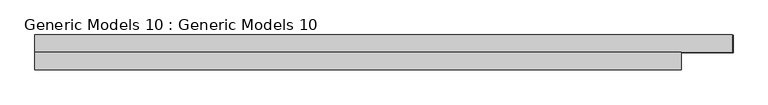
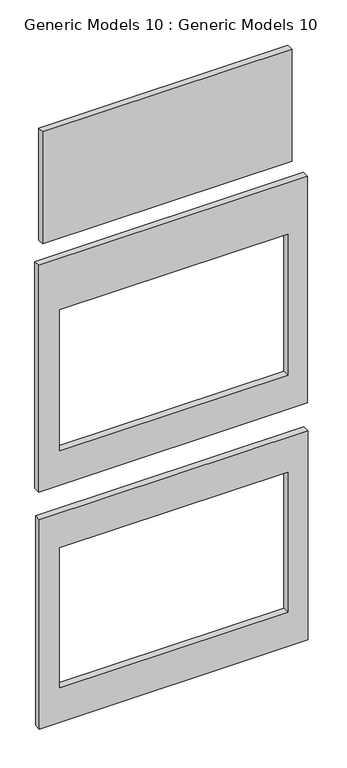
"""IFC4 building model written with IfcOpenShell, lengths in millimetres: proxy geometry, Generic Models 10 : Generic Models 10."""

from ifc_helpers import new_model, si_unit, frame, origin, place, context, project, spatial, polyline, outline, extrude, source, transform, mapped, element, save


def generic_models_10_generic_models_10_e6df43e6(model_context):
    return source(origin(), model_context, "Body", "SweptSolid", [
        extrude(outline(polyline([(-13111.1695233, -14337.9752569), (-15938.4468823, -14337.9752569), (-15938.4468823, -14261.7752569), (-13111.1695233, -14261.7752569), (-13111.1695233, -14337.9752569)])), frame((0.0, 0.0, 9448.8), z_axis=(0.0, 0.0, 1.0), x_axis=(1.0, 0.0, 0.0)), (0.0, 0.0, 1.0), 1341.7282636),
        extrude(outline(polyline([(6096.0, -12884.8411453), (6096.0, -15930.5695233), (3588.5355704, -15930.5695233), (3588.5355704, -12884.8411453), (6096.0, -12884.8411453)]), holes=[polyline([(5678.6814593, -13111.1695233), (4001.8016497, -13111.1695233), (4001.8016497, -15701.9695233), (5678.6814593, -15701.9695233), (5678.6814593, -13111.1695233)])]), frame((0.0, -14261.7752569, 0.0), z_axis=(0.0, 1.0, 0.0), x_axis=(0.0, 0.0, 1.0)), (0.0, 0.0, 1.0), 76.2),
        extrude(outline(polyline([(6429.1436541, -12889.569466), (9144.0, -12889.569466), (9144.0, -15938.4468823), (6429.1436541, -15938.4468823), (6429.1436541, -12889.569466)]), holes=[polyline([(8530.8973501, -13111.1695233), (6841.9204311, -13111.1695233), (6841.9204311, -15701.9695233), (8530.8973501, -15701.9695233), (8530.8973501, -13111.1695233)])]), frame((0.0, -14261.7752569, 0.0), z_axis=(0.0, 1.0, 0.0), x_axis=(0.0, 0.0, 1.0)), (0.0, 0.0, 1.0), 76.2),
    ])


if __name__ == "__main__":
    model = new_model("IFC4")
    model_context = context("Model", 3, world=origin())
    ifc_project = project(units=[si_unit("LENGTHUNIT", "METRE", prefix="MILLI")], contexts=[model_context])
    site = spatial("IfcSite", under=ifc_project)
    building = spatial("IfcBuilding", under=site)
    placement = place(None, origin())
    generic_models_10_generic_models_10_shape = generic_models_10_generic_models_10_e6df43e6(model_context)
    element("IfcBuildingElementProxy", 1, Name="Generic Models 10 : Generic Models 10", ObjectType="Generic Models 10 : Generic Models 10", at=placement, inside=building, context=model_context, shape_type="MappedRepresentation", body=[
        mapped(generic_models_10_generic_models_10_shape, transform((0.0, 0.0, 0.0), x_axis=(1.0, 0.0, 0.0), y_axis=(0.0, 1.0, 0.0), z_axis=(0.0, 0.0, 1.0))),
    ])
    save(model, "model.ifc")
